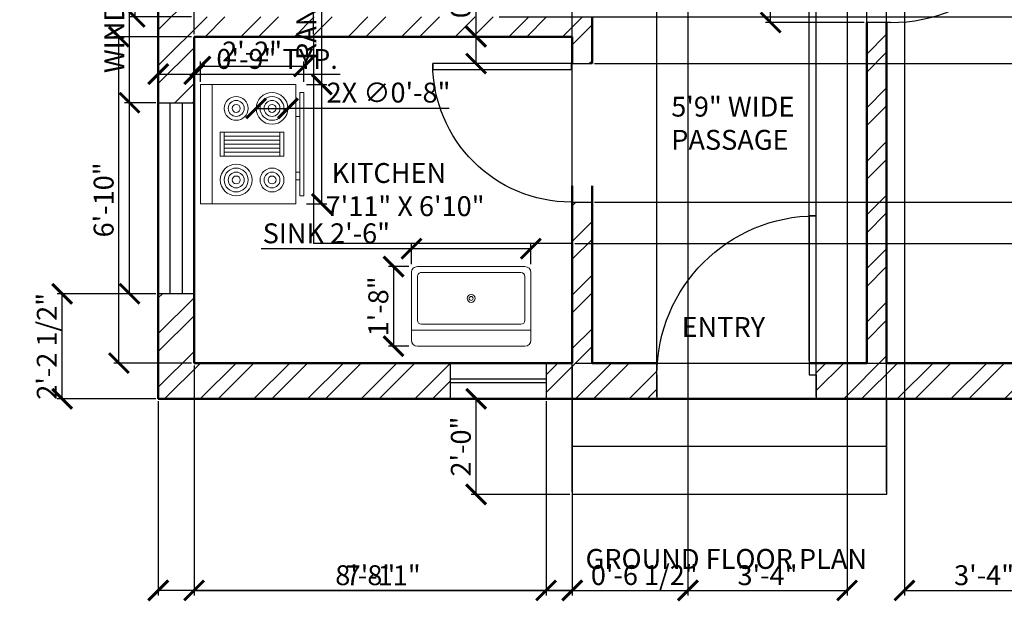
# Model space of a CAD drawing. Units: inches. Extents: x 683 to 1274, y 1901 to 2385.
# Tile 1 of 5: x 683 to 930, y 1901 to 2049. Entities that reach past the tile are written whole.
import ezdxf

# ---------------------------------------------------------------- set-up
doc = ezdxf.new("R2010")
doc.units = ezdxf.units.IN
for name, color, linetype, lineweight in [('A-AREA-IDEN', 3, 'Continuous', 25), ('A-EQPM', 2, 'Continuous', 18), ('A-FLOR-CASE', 2, 'Continuous', 25), ('A-FLOR-FIXT', 2, 'Continuous', 18), ('A-FLOR-STRS', 7, 'Continuous', 25), ('A-WALL-PATT', 8, 'Continuous', 13), ('DIM', 3, 'Continuous', 18), ('DOORS', 4, 'Continuous', 25), ('TEXT', 1, 'Continuous', 25), ('VENTILATOR', 11, 'Continuous', 25), ('walls', 6, 'Continuous', 50), ('WINDOWS', 30, 'Continuous', 25)]:
    doc.layers.add(name, color=color, linetype=linetype, lineweight=lineweight)
doc.styles.get("Standard").update_dxf_attribs({"font": 'arial.ttf'})
doc.dimstyles.new('ISO-25', dxfattribs={"dimtxt": 5, "dimasz": 5, "dimexe": 1.25, "dimexo": 0.625, "dimtad": 1, "dimdec": 1, "dimlunit": 4, "dimtxsty": 'Standard', "dimblk": 'ARCHTICK', "dimcen": 2.5, "dimadec": 0, "dimazin": 0, "dimtfac": 1, "dimtdec": 1, "dimtmove": 0, "dimatfit": 3, "dimfxl": 1, "dimarcsym": 0})

# ---------------------------------------------------------------- blocks, each defined once
blk = doc.blocks.new('Range-Oven - 30 in top')
for p, q in [((0, -3), (30, -3)), ((12, -6), (18, -6)), ((13, -20), (13, -6)), ((14, -6), (14, -20)), ((15, -20), (15, -6)), ((16, -6), (16, -20)), ((17, -20), (17, -6)), ((18, -20), (12, -20)), ((6, -24), (6, -25)), ((8, -25), (8, -24)), ((22, -25), (22, -24)), ((24, -24), (24, -25))]:
    blk.add_line(p, q)
for points in [[(0, -24), (0, 0), (30, 0), (30, -24)], [(12, -21), (12, -5), (18, -5), (18, -21)], [(2, -26), (2, -25), (28, -25), (28, -26)]]:
    blk.add_lwpolyline(points, close=True)
for centre, radius in [((6, -9), 4), ((6, -9), 3), ((6, -9), 2), ((24, -9), 3), ((24, -9), 2), ((6, -9), 1), ((24, -9), 1), ((24, -18), 4), ((6, -18), 3), ((6, -18), 2), ((6, -18), 1), ((24, -18), 3), ((24, -18), 2), ((24, -18), 1)]:
    blk.add_circle(centre, radius)
blk = doc.blocks.new('Sink-single - 30 in top')
blk.add_line((-15, -3.999996), (15, -3.999996))
for points in [[(-13.5, 0), (13.5, 0)], [(-15, -18.499996), (-15, -1.5)], [(15, -1.5), (15, -18.499996)], [(-13.5, -17.499996), (-13.5, -6.499996)], [(-12.5, -5.499996), (12.5, -5.499996)], [(13.5, -6.499996), (13.5, -17.499996)], [(12.5, -18.499996), (-12.5, -18.499996)], [(13.5, -19.999996), (-13.5, -19.999996)]]:
    blk.add_lwpolyline(points)
for radius in [1, 0.5]:
    blk.add_circle((0, -11.999996), radius)
for centre, radius, start, end in [((-13.5, -1.5), 1.5, 90, 180), ((13.5, -1.5), 1.5, 0, 90), ((-12.5, -6.499996), 1, 90, 180), ((12.5, -6.499996), 1, 0, 90), ((-13.5, -18.499996), 1.5, 180, 270), ((-12.5, -17.499996), 1, 180, 270), ((12.5, -17.499996), 1, 270, 0), ((13.5, -18.499996), 1.5, 270, 0)]:
    blk.add_arc(centre, radius, start, end)
blk = doc.blocks.new('VENTILATOR')
at = {"layer": 'VENTILATOR'}
for p, q in [((1084.96, 2166.43), (1093.96, 2166.43)), ((1084.96, 2142.43), (1084.96, 2166.43)), ((1088.96, 2142.43), (1088.96, 2166.43)), ((1089.96, 2166.43), (1089.96, 2142.43)), ((1093.96, 2166.43), (1093.96, 2142.43)), ((1093.96, 2142.43), (1084.96, 2142.43))]:
    blk.add_line(p, q, dxfattribs=at)
blk = doc.blocks.new('W2')
at = {"layer": 'WINDOWS'}
for p, q in [((1126.75, 2245.25), (1135.75, 2245.25)), ((1126.75, 2197.25), (1126.75, 2245.25)), ((1129.75, 2197.25), (1129.75, 2245.25)), ((1132.75, 2245.25), (1132.75, 2197.25)), ((1135.75, 2245.25), (1135.75, 2197.25)), ((1135.75, 2197.25), (1126.75, 2197.25))]:
    blk.add_line(p, q, dxfattribs=at)
blk = doc.blocks.new('*U18')
for p, q in [((0, 0), (0, -6)), ((40, 0), (40, -6))]:
    blk.add_line(p, q)
blk.add_lwpolyline([(0, 0), (0, 40), (1.75, 40), (1.75, 0)], close=True)
blk.add_arc((0, 0), 40, 0, 90)
blk = doc.blocks.new('_ArchTick')
at = {"color": 0, "linetype": 'ByBlock', "const_width": 0.15}
blk.add_lwpolyline([(-0.5, -0.5), (0.5, 0.5)], dxfattribs=at)
blk = doc.blocks.new('*D23')
at = {"layer": 'Defpoints', "color": 0, "transparency": 16777216}
for p in [(726.42, 2191.78), (711.49, 2049.78), (726.42, 2049.78)]:
    blk.add_point(p, dxfattribs=at)
at = {"layer": 'DIM', "color": 0, "lineweight": -2, "transparency": 16777216}
for p, q in [((725.79, 2191.78), (710.24, 2191.78)), ((711.49, 2191.78), (711.49, 2049.78)), ((725.79, 2049.78), (710.24, 2049.78))]:
    blk.add_line(p, q, dxfattribs=at)
at = {"layer": 'DIM', "color": 0, "lineweight": -2, "transparency": 16777216, "xscale": 5, "yscale": 5, "zscale": 5}
for p, rotation in [((711.49, 2191.78), 90), ((711.49, 2049.78), 270)]:
    blk.add_blockref('_ArchTick', p, dxfattribs=dict(at, rotation=rotation))
at = {"layer": 'DIM', "color": 0, "transparency": 16777216, "insert": (708.32, 2120.78), "char_height": 5, "attachment_point": 5, "rotation": 90}
blk.add_mtext('11\'-10"', dxfattribs=at)
blk = doc.blocks.new('*D24')
at = {"layer": 'Defpoints', "color": 0, "transparency": 16777216}
for p in [(707.52, 2044.78), (726.42, 2044.78), (726.42, 1962.78)]:
    blk.add_point(p, dxfattribs=at)
at = {"layer": 'DIM', "color": 0, "lineweight": -2, "transparency": 16777216}
for p, q in [((725.79, 2044.78), (706.27, 2044.78)), ((707.52, 1962.78), (707.52, 2044.78)), ((725.79, 1962.78), (706.27, 1962.78))]:
    blk.add_line(p, q, dxfattribs=at)
at = {"layer": 'DIM', "color": 0, "lineweight": -2, "transparency": 16777216, "xscale": 5, "yscale": 5, "zscale": 5}
for p, rotation in [((707.52, 2044.78), 90), ((707.52, 1962.78), 270)]:
    blk.add_blockref('_ArchTick', p, dxfattribs=dict(at, rotation=rotation))
at = {"layer": 'DIM', "color": 0, "transparency": 16777216, "insert": (704.34, 2003.78), "char_height": 5, "attachment_point": 5, "rotation": 90}
blk.add_mtext('6\'-10"', dxfattribs=at)
blk = doc.blocks.new('*D29')
at = {"layer": 'Defpoints', "color": 0, "transparency": 16777216}
for p in [(710.22, 2028.18), (717.42, 2028.18), (717.42, 1980.18)]:
    blk.add_point(p, dxfattribs=at)
at = {"layer": 'DIM', "color": 0, "lineweight": -2, "transparency": 16777216}
for p, q in [((710.22, 2028.18), (710.22, 2110.12)), ((716.79, 2028.18), (708.97, 2028.18)), ((710.22, 1980.18), (710.22, 2028.18)), ((716.79, 1980.18), (708.97, 1980.18))]:
    blk.add_line(p, q, dxfattribs=at)
at = {"layer": 'DIM', "color": 0, "lineweight": -2, "transparency": 16777216, "xscale": 5, "yscale": 5, "zscale": 5}
for p, rotation in [((710.22, 2028.18), 90), ((710.22, 1980.18), 270)]:
    blk.add_blockref('_ArchTick', p, dxfattribs=dict(at, rotation=rotation))
at = {"layer": 'DIM', "color": 0, "transparency": 16777216, "insert": (707.01, 2071.65), "char_height": 5, "attachment_point": 5, "rotation": 90}
blk.add_mtext('WINDOW W2 4\'-0" TYP.', dxfattribs=at)
blk = doc.blocks.new('*D30')
at = {"layer": 'Defpoints', "color": 0, "transparency": 16777216}
for p in [(726.42, 2035.38), (717.42, 2028.18), (726.42, 2028.18)]:
    blk.add_point(p, dxfattribs=at)
at = {"layer": 'DIM', "color": 0, "lineweight": -2, "transparency": 16777216}
for p, q in [((717.42, 2028.81), (717.42, 2036.63)), ((726.42, 2028.81), (726.42, 2036.63)), ((717.42, 2035.38), (726.42, 2035.38)), ((726.42, 2035.38), (763.15, 2035.38))]:
    blk.add_line(p, q, dxfattribs=at)
at = {"layer": 'DIM', "color": 0, "lineweight": -2, "transparency": 16777216, "xscale": 5, "yscale": 5, "zscale": 5, "rotation": 180}
blk.add_blockref('_ArchTick', (717.42, 2035.38), dxfattribs=at)
at = {"layer": 'DIM', "color": 0, "lineweight": -2, "transparency": 16777216, "xscale": 5, "yscale": 5, "zscale": 5}
blk.add_blockref('_ArchTick', (726.42, 2035.38), dxfattribs=at)
at = {"layer": 'DIM', "color": 0, "transparency": 16777216, "insert": (747.28, 2038.56), "char_height": 5, "attachment_point": 5}
blk.add_mtext('0\'-9" TYP.', dxfattribs=at)
blk = doc.blocks.new('*D33')
at = {"layer": 'Defpoints', "color": 0, "transparency": 16777216}
for p in [(754, 2032.78), (758.5, 2032.78), (754, 2002.78)]:
    blk.add_point(p, dxfattribs=at)
at = {"layer": 'DIM', "color": 0, "lineweight": -2, "transparency": 16777216}
for p, q in [((758.5, 2032.78), (758.5, 2078.84)), ((754.63, 2032.78), (759.75, 2032.78)), ((758.5, 2002.78), (758.5, 2032.78)), ((754.63, 2002.78), (759.75, 2002.78))]:
    blk.add_line(p, q, dxfattribs=at)
at = {"layer": 'DIM', "color": 0, "lineweight": -2, "transparency": 16777216, "xscale": 5, "yscale": 5, "zscale": 5}
for p, rotation in [((758.5, 2032.78), 90), ((758.5, 2002.78), 270)]:
    blk.add_blockref('_ArchTick', p, dxfattribs=dict(at, rotation=rotation))
at = {"layer": 'DIM', "color": 0, "transparency": 16777216, "insert": (755.29, 2058.31), "char_height": 5, "attachment_point": 5, "rotation": 90}
blk.add_mtext('RANGE 2\'-6"', dxfattribs=at)
blk = doc.blocks.new('*D34')
at = {"layer": 'Defpoints', "color": 0, "transparency": 16777216}
for p in [(728, 2037.28), (728, 2032.78), (754, 2032.78)]:
    blk.add_point(p, dxfattribs=at)
at = {"layer": 'DIM', "color": 0, "lineweight": -2, "transparency": 16777216}
for p, q in [((728, 2033.41), (728, 2038.53)), ((754, 2033.41), (754, 2038.53)), ((754, 2037.28), (728, 2037.28))]:
    blk.add_line(p, q, dxfattribs=at)
at = {"layer": 'DIM', "color": 0, "lineweight": -2, "transparency": 16777216, "xscale": 5, "yscale": 5, "zscale": 5, "rotation": 180}
blk.add_blockref('_ArchTick', (728, 2037.28), dxfattribs=at)
at = {"layer": 'DIM', "color": 0, "lineweight": -2, "transparency": 16777216, "xscale": 5, "yscale": 5, "zscale": 5}
blk.add_blockref('_ArchTick', (754, 2037.28), dxfattribs=at)
at = {"layer": 'DIM', "color": 0, "transparency": 16777216, "insert": (741, 2040.42), "char_height": 5, "attachment_point": 5}
blk.add_mtext('2\'-2"', dxfattribs=at)
blk = doc.blocks.new('*D35')
at = {"layer": 'Defpoints', "color": 0, "transparency": 16777216}
for p in [(781.03, 1991.52), (781.03, 1987.02), (811.03, 1987.02)]:
    blk.add_point(p, dxfattribs=at)
at = {"layer": 'DIM', "color": 0, "lineweight": -2, "transparency": 16777216}
for p, q in [((781.03, 1991.52), (743.27, 1991.52)), ((781.03, 1987.65), (781.03, 1992.77)), ((811.03, 1991.52), (781.03, 1991.52)), ((811.03, 1987.65), (811.03, 1992.77))]:
    blk.add_line(p, q, dxfattribs=at)
at = {"layer": 'DIM', "color": 0, "lineweight": -2, "transparency": 16777216, "xscale": 5, "yscale": 5, "zscale": 5, "rotation": 180}
blk.add_blockref('_ArchTick', (781.03, 1991.52), dxfattribs=at)
at = {"layer": 'DIM', "color": 0, "lineweight": -2, "transparency": 16777216, "xscale": 5, "yscale": 5, "zscale": 5}
blk.add_blockref('_ArchTick', (811.03, 1991.52), dxfattribs=at)
at = {"layer": 'DIM', "color": 0, "transparency": 16777216, "insert": (759.65, 1994.73), "char_height": 5, "attachment_point": 5}
blk.add_mtext('SINK 2\'-6"', dxfattribs=at)
blk = doc.blocks.new('*D36')
at = {"layer": 'Defpoints', "color": 0, "transparency": 16777216}
for p in [(781.03, 1987.02), (776.53, 1967.02), (781.03, 1967.02)]:
    blk.add_point(p, dxfattribs=at)
at = {"layer": 'DIM', "color": 0, "lineweight": -2, "transparency": 16777216}
for p, q in [((780.41, 1987.02), (775.28, 1987.02)), ((776.53, 1987.02), (776.53, 1967.02)), ((780.41, 1967.02), (775.28, 1967.02))]:
    blk.add_line(p, q, dxfattribs=at)
at = {"layer": 'DIM', "color": 0, "lineweight": -2, "transparency": 16777216, "xscale": 5, "yscale": 5, "zscale": 5}
for p, rotation in [((776.53, 1987.02), 90), ((776.53, 1967.02), 270)]:
    blk.add_blockref('_ArchTick', p, dxfattribs=dict(at, rotation=rotation))
at = {"layer": 'DIM', "color": 0, "transparency": 16777216, "insert": (773.35, 1977.02), "char_height": 5, "attachment_point": 5, "rotation": 90}
blk.add_mtext('1\'-8"', dxfattribs=at)
blk = doc.blocks.new('*D39')
at = {"layer": 'Defpoints', "color": 0, "transparency": 16777216}
for p in [(900.42, 2361.93), (821.42, 1929.78), (900.42, 1929.78)]:
    blk.add_point(p, dxfattribs=at)
at = {"layer": 'DIM', "color": 0, "lineweight": -2, "transparency": 16777216}
for p, q in [((821.42, 1930.41), (821.42, 2363.18)), ((900.42, 1930.41), (900.42, 2363.18)), ((821.42, 2361.93), (900.42, 2361.93))]:
    blk.add_line(p, q, dxfattribs=at)
at = {"layer": 'DIM', "color": 0, "lineweight": -2, "transparency": 16777216, "xscale": 5, "yscale": 5, "zscale": 5, "rotation": 180}
blk.add_blockref('_ArchTick', (821.42, 2361.93), dxfattribs=at)
at = {"layer": 'DIM', "color": 0, "lineweight": -2, "transparency": 16777216, "xscale": 5, "yscale": 5, "zscale": 5}
blk.add_blockref('_ArchTick', (900.42, 2361.93), dxfattribs=at)
at = {"layer": 'DIM', "color": 0, "transparency": 16777216, "insert": (860.92, 2365.11), "char_height": 5, "attachment_point": 5}
blk.add_mtext('6\'-7"', dxfattribs=at)
blk = doc.blocks.new('*D40')
at = {"layer": 'Defpoints', "color": 0, "transparency": 16777216}
for p in [(797.27, 1953.78), (821.42, 1953.78), (821.42, 1929.78)]:
    blk.add_point(p, dxfattribs=at)
at = {"layer": 'DIM', "color": 0, "lineweight": -2, "transparency": 16777216}
for p, q in [((820.79, 1953.78), (796.02, 1953.78)), ((797.27, 1929.78), (797.27, 1953.78)), ((820.79, 1929.78), (796.02, 1929.78))]:
    blk.add_line(p, q, dxfattribs=at)
at = {"layer": 'DIM', "color": 0, "lineweight": -2, "transparency": 16777216, "xscale": 5, "yscale": 5, "zscale": 5}
for p, rotation in [((797.27, 1953.78), 90), ((797.27, 1929.78), 270)]:
    blk.add_blockref('_ArchTick', p, dxfattribs=dict(at, rotation=rotation))
at = {"layer": 'DIM', "color": 0, "transparency": 16777216, "insert": (794.09, 1941.78), "char_height": 5, "attachment_point": 5, "rotation": 90}
blk.add_mtext('2\'-0"', dxfattribs=at)
blk = doc.blocks.new('*D41')
at = {"layer": 'Defpoints', "color": 0, "transparency": 16777216}
for p in [(726.42, 1962.78), (821.42, 1962.78), (821.42, 1905.63)]:
    blk.add_point(p, dxfattribs=at)
at = {"layer": 'DIM', "color": 0, "lineweight": -2, "transparency": 16777216}
for p, q in [((726.42, 1962.16), (726.42, 1904.38)), ((821.42, 1962.16), (821.42, 1904.38)), ((726.42, 1905.63), (821.42, 1905.63))]:
    blk.add_line(p, q, dxfattribs=at)
at = {"layer": 'DIM', "color": 0, "lineweight": -2, "transparency": 16777216, "xscale": 5, "yscale": 5, "zscale": 5, "rotation": 180}
blk.add_blockref('_ArchTick', (726.42, 1905.63), dxfattribs=at)
at = {"layer": 'DIM', "color": 0, "lineweight": -2, "transparency": 16777216, "xscale": 5, "yscale": 5, "zscale": 5}
blk.add_blockref('_ArchTick', (821.42, 1905.63), dxfattribs=at)
at = {"layer": 'DIM', "color": 0, "transparency": 16777216, "insert": (773.92, 1908.77), "char_height": 5, "attachment_point": 5}
blk.add_mtext('7\'-11"', dxfattribs=at)
blk = doc.blocks.new('*D42')
at = {"layer": 'Defpoints', "color": 0, "transparency": 16777216}
for p in [(826.42, 2038.04), (826.42, 2003.23), (1053.57, 2003.23)]:
    blk.add_point(p, dxfattribs=at)
at = {"layer": 'DIM', "color": 0, "lineweight": -2, "transparency": 16777216}
for p, q in [((827.04, 2038.04), (1054.82, 2038.04)), ((1053.57, 2038.04), (1053.57, 2003.23)), ((827.04, 2003.23), (1054.82, 2003.23))]:
    blk.add_line(p, q, dxfattribs=at)
at = {"layer": 'DIM', "color": 0, "lineweight": -2, "transparency": 16777216, "xscale": 5, "yscale": 5, "zscale": 5}
for p, rotation in [((1053.57, 2038.04), 90), ((1053.57, 2003.23), 270)]:
    blk.add_blockref('_ArchTick', p, dxfattribs=dict(at, rotation=rotation))
at = {"layer": 'DIM', "color": 0, "transparency": 16777216, "insert": (1050.43, 2020.64), "char_height": 5, "attachment_point": 5, "rotation": 90}
blk.add_mtext('2\'-11"', dxfattribs=at)
blk = doc.blocks.new('*D44')
at = {"layer": 'Defpoints', "color": 0, "transparency": 16777216}
for p in [(882.7, 2361.93), (842.7, 1953.78), (882.7, 1953.78)]:
    blk.add_point(p, dxfattribs=at)
at = {"layer": 'DIM', "color": 0, "lineweight": -2, "transparency": 16777216}
for p, q in [((842.7, 1954.41), (842.7, 2363.18)), ((882.7, 1954.41), (882.7, 2363.18)), ((842.7, 2361.93), (882.7, 2361.93))]:
    blk.add_line(p, q, dxfattribs=at)
at = {"layer": 'DIM', "color": 0, "lineweight": -2, "transparency": 16777216, "xscale": 5, "yscale": 5, "zscale": 5, "rotation": 180}
blk.add_blockref('_ArchTick', (842.7, 2361.93), dxfattribs=at)
at = {"layer": 'DIM', "color": 0, "lineweight": -2, "transparency": 16777216, "xscale": 5, "yscale": 5, "zscale": 5}
blk.add_blockref('_ArchTick', (882.7, 2361.93), dxfattribs=at)
at = {"layer": 'DIM', "color": 0, "transparency": 16777216, "insert": (862.7, 2365.11), "char_height": 5, "attachment_point": 5}
blk.add_mtext('3\'-4"', dxfattribs=at)
blk = doc.blocks.new('*D45')
at = {"layer": 'Defpoints', "color": 0, "transparency": 16777216}
for p in [(850.48, 2191.78), (890.48, 2191.78), (890.48, 1905.63)]:
    blk.add_point(p, dxfattribs=at)
at = {"layer": 'DIM', "color": 0, "lineweight": -2, "transparency": 16777216}
for p, q in [((850.48, 2191.16), (850.48, 1904.38)), ((890.48, 2191.16), (890.48, 1904.38)), ((850.48, 1905.63), (890.48, 1905.63))]:
    blk.add_line(p, q, dxfattribs=at)
at = {"layer": 'DIM', "color": 0, "lineweight": -2, "transparency": 16777216, "xscale": 5, "yscale": 5, "zscale": 5, "rotation": 180}
blk.add_blockref('_ArchTick', (850.48, 1905.63), dxfattribs=at)
at = {"layer": 'DIM', "color": 0, "lineweight": -2, "transparency": 16777216, "xscale": 5, "yscale": 5, "zscale": 5}
blk.add_blockref('_ArchTick', (890.48, 1905.63), dxfattribs=at)
at = {"layer": 'DIM', "color": 0, "transparency": 16777216, "insert": (870.48, 1908.81), "char_height": 5, "attachment_point": 5}
blk.add_mtext('3\'-4"', dxfattribs=at)
blk = doc.blocks.new('*D46')
at = {"layer": 'Defpoints', "color": 0, "transparency": 16777216}
for p in [(904.89, 2191.78), (944.89, 2191.78), (944.89, 1905.63)]:
    blk.add_point(p, dxfattribs=at)
at = {"layer": 'DIM', "color": 0, "lineweight": -2, "transparency": 16777216}
for p, q in [((904.89, 2191.16), (904.89, 1904.38)), ((944.89, 2191.16), (944.89, 1904.38)), ((904.89, 1905.63), (944.89, 1905.63))]:
    blk.add_line(p, q, dxfattribs=at)
at = {"layer": 'DIM', "color": 0, "lineweight": -2, "transparency": 16777216, "xscale": 5, "yscale": 5, "zscale": 5, "rotation": 180}
blk.add_blockref('_ArchTick', (904.89, 1905.63), dxfattribs=at)
at = {"layer": 'DIM', "color": 0, "lineweight": -2, "transparency": 16777216, "xscale": 5, "yscale": 5, "zscale": 5}
blk.add_blockref('_ArchTick', (944.89, 1905.63), dxfattribs=at)
at = {"layer": 'DIM', "color": 0, "transparency": 16777216, "insert": (924.89, 1908.81), "char_height": 5, "attachment_point": 5}
blk.add_mtext('3\'-4"', dxfattribs=at)
blk = doc.blocks.new('*D47')
at = {"layer": 'Defpoints', "color": 0, "transparency": 16777216}
for p in [(871.27, 2088.36), (895.42, 2088.36), (895.42, 2048.36)]:
    blk.add_point(p, dxfattribs=at)
at = {"layer": 'DIM', "color": 0, "lineweight": -2, "transparency": 16777216}
for p, q in [((894.79, 2088.36), (870.02, 2088.36)), ((871.27, 2048.36), (871.27, 2088.36)), ((894.79, 2048.36), (870.02, 2048.36))]:
    blk.add_line(p, q, dxfattribs=at)
at = {"layer": 'DIM', "color": 0, "lineweight": -2, "transparency": 16777216, "xscale": 5, "yscale": 5, "zscale": 5}
for p, rotation in [((871.27, 2088.36), 90), ((871.27, 2048.36), 270)]:
    blk.add_blockref('_ArchTick', p, dxfattribs=dict(at, rotation=rotation))
at = {"layer": 'DIM', "color": 0, "transparency": 16777216, "insert": (868.09, 2068.36), "char_height": 5, "attachment_point": 5, "rotation": 90}
blk.add_mtext('3\'-4"', dxfattribs=at)
blk = doc.blocks.new('*D49')
at = {"layer": 'Defpoints', "color": 0, "transparency": 16777216}
for p in [(802.42, 2085.78), (1053.57, 2085.78), (802.42, 2049.78)]:
    blk.add_point(p, dxfattribs=at)
at = {"layer": 'DIM', "color": 0, "lineweight": -2, "transparency": 16777216}
for p, q in [((803.04, 2085.78), (1054.82, 2085.78)), ((1053.57, 2049.78), (1053.57, 2085.78)), ((803.04, 2049.78), (1054.82, 2049.78))]:
    blk.add_line(p, q, dxfattribs=at)
at = {"layer": 'DIM', "color": 0, "lineweight": -2, "transparency": 16777216, "xscale": 5, "yscale": 5, "zscale": 5}
for p, rotation in [((1053.57, 2085.78), 90), ((1053.57, 2049.78), 270)]:
    blk.add_blockref('_ArchTick', p, dxfattribs=dict(at, rotation=rotation))
at = {"layer": 'DIM', "color": 0, "transparency": 16777216, "insert": (1050.39, 2067.78), "char_height": 5, "attachment_point": 5, "rotation": 90}
blk.add_mtext('3\'-0"', dxfattribs=at)
blk = doc.blocks.new('*D56')
at = {"layer": 'Defpoints', "color": 0, "transparency": 16777216}
for p in [(693.27, 1980.18), (717.42, 1980.18), (717.42, 1953.78)]:
    blk.add_point(p, dxfattribs=at)
at = {"layer": 'DIM', "color": 0, "lineweight": -2, "transparency": 16777216}
for p, q in [((716.79, 1980.18), (692.02, 1980.18)), ((693.27, 1953.78), (693.27, 1980.18)), ((716.79, 1953.78), (692.02, 1953.78))]:
    blk.add_line(p, q, dxfattribs=at)
at = {"layer": 'DIM', "color": 0, "lineweight": -2, "transparency": 16777216, "xscale": 5, "yscale": 5, "zscale": 5}
for p, rotation in [((693.27, 1980.18), 90), ((693.27, 1953.78), 270)]:
    blk.add_blockref('_ArchTick', p, dxfattribs=dict(at, rotation=rotation))
at = {"layer": 'DIM', "color": 0, "transparency": 16777216, "insert": (690.06, 1966.98), "char_height": 5, "attachment_point": 5, "rotation": 90}
blk.add_mtext('2\'-2 1/2"', dxfattribs=at)
blk = doc.blocks.new('*D57')
at = {"layer": 'Defpoints', "color": 0, "transparency": 16777216}
for p in [(814.86, 1953.78), (821.42, 1953.78), (821.42, 1905.63)]:
    blk.add_point(p, dxfattribs=at)
at = {"layer": 'DIM', "color": 0, "lineweight": -2, "transparency": 16777216}
for p, q in [((814.86, 1953.16), (814.86, 1904.38)), ((821.42, 1953.16), (821.42, 1904.38)), ((814.86, 1905.63), (821.42, 1905.63)), ((821.42, 1905.63), (852.61, 1905.63))]:
    blk.add_line(p, q, dxfattribs=at)
at = {"layer": 'DIM', "color": 0, "lineweight": -2, "transparency": 16777216, "xscale": 5, "yscale": 5, "zscale": 5, "rotation": 180}
blk.add_blockref('_ArchTick', (814.86, 1905.63), dxfattribs=at)
at = {"layer": 'DIM', "color": 0, "lineweight": -2, "transparency": 16777216, "xscale": 5, "yscale": 5, "zscale": 5}
blk.add_blockref('_ArchTick', (821.42, 1905.63), dxfattribs=at)
at = {"layer": 'DIM', "color": 0, "transparency": 16777216, "insert": (839.52, 1908.84), "char_height": 5, "attachment_point": 5}
blk.add_mtext('0\'-6 1/2"', dxfattribs=at)
blk = doc.blocks.new('*D58')
at = {"layer": 'Defpoints', "color": 0, "transparency": 16777216}
for p in [(756.42, 2361.93), (726.42, 2044.78), (756.42, 2044.78)]:
    blk.add_point(p, dxfattribs=at)
at = {"layer": 'DIM', "color": 0, "lineweight": -2, "transparency": 16777216}
for p, q in [((726.42, 2045.41), (726.42, 2363.18)), ((756.42, 2045.41), (756.42, 2363.18)), ((726.42, 2361.93), (756.42, 2361.93))]:
    blk.add_line(p, q, dxfattribs=at)
at = {"layer": 'DIM', "color": 0, "lineweight": -2, "transparency": 16777216, "xscale": 5, "yscale": 5, "zscale": 5, "rotation": 180}
blk.add_blockref('_ArchTick', (726.42, 2361.93), dxfattribs=at)
at = {"layer": 'DIM', "color": 0, "lineweight": -2, "transparency": 16777216, "xscale": 5, "yscale": 5, "zscale": 5}
blk.add_blockref('_ArchTick', (756.42, 2361.93), dxfattribs=at)
at = {"layer": 'DIM', "color": 0, "transparency": 16777216, "insert": (741.42, 2365.11), "char_height": 5, "attachment_point": 5}
blk.add_mtext('2\'-6"', dxfattribs=at)
blk = doc.blocks.new('*D59')
at = {"layer": 'Defpoints', "color": 0, "transparency": 16777216}
for p in [(821.42, 1992.78), (821.42, 1962.78), (1053.57, 1962.78)]:
    blk.add_point(p, dxfattribs=at)
at = {"layer": 'DIM', "color": 0, "lineweight": -2, "transparency": 16777216}
for p, q in [((822.04, 1992.78), (1054.82, 1992.78)), ((1053.57, 1992.78), (1053.57, 1962.78)), ((822.04, 1962.78), (1054.82, 1962.78))]:
    blk.add_line(p, q, dxfattribs=at)
at = {"layer": 'DIM', "color": 0, "lineweight": -2, "transparency": 16777216, "xscale": 5, "yscale": 5, "zscale": 5}
for p, rotation in [((1053.57, 1992.78), 90), ((1053.57, 1962.78), 270)]:
    blk.add_blockref('_ArchTick', p, dxfattribs=dict(at, rotation=rotation))
at = {"layer": 'DIM', "color": 0, "transparency": 16777216, "insert": (1050.39, 1977.78), "char_height": 5, "attachment_point": 5, "rotation": 90}
blk.add_mtext('2\'-6"', dxfattribs=at)
blk = doc.blocks.new('*D61')
at = {"layer": 'Defpoints', "color": 0, "transparency": 16777216}
for p in [(895.42, 2361.93), (880.95, 1962.78), (895.42, 1962.78)]:
    blk.add_point(p, dxfattribs=at)
at = {"layer": 'DIM', "color": 0, "lineweight": -2, "transparency": 16777216}
for p, q in [((880.95, 1963.41), (880.95, 2363.18)), ((895.42, 1963.41), (895.42, 2363.18)), ((880.95, 2361.93), (895.42, 2361.93)), ((895.42, 2361.93), (926.14, 2361.93))]:
    blk.add_line(p, q, dxfattribs=at)
at = {"layer": 'DIM', "color": 0, "lineweight": -2, "transparency": 16777216, "xscale": 5, "yscale": 5, "zscale": 5, "rotation": 180}
blk.add_blockref('_ArchTick', (880.95, 2361.93), dxfattribs=at)
at = {"layer": 'DIM', "color": 0, "lineweight": -2, "transparency": 16777216, "xscale": 5, "yscale": 5, "zscale": 5}
blk.add_blockref('_ArchTick', (895.42, 2361.93), dxfattribs=at)
at = {"layer": 'DIM', "color": 0, "transparency": 16777216, "insert": (913.28, 2365.14), "char_height": 5, "attachment_point": 5}
blk.add_mtext('1\'-2 1/2"', dxfattribs=at)
blk = doc.blocks.new('*D62')
at = {"layer": 'Defpoints', "color": 0, "transparency": 16777216}
for p in [(717.42, 1953.78), (821.42, 1929.78), (717.42, 1905.63)]:
    blk.add_point(p, dxfattribs=at)
at = {"layer": 'DIM', "color": 0, "lineweight": -2, "transparency": 16777216}
for p, q in [((717.42, 1953.16), (717.42, 1904.38)), ((821.42, 1929.16), (821.42, 1904.38)), ((821.42, 1905.63), (717.42, 1905.63))]:
    blk.add_line(p, q, dxfattribs=at)
at = {"layer": 'DIM', "color": 0, "lineweight": -2, "transparency": 16777216, "xscale": 5, "yscale": 5, "zscale": 5, "rotation": 180}
blk.add_blockref('_ArchTick', (717.42, 1905.63), dxfattribs=at)
at = {"layer": 'DIM', "color": 0, "lineweight": -2, "transparency": 16777216, "xscale": 5, "yscale": 5, "zscale": 5}
blk.add_blockref('_ArchTick', (821.42, 1905.63), dxfattribs=at)
at = {"layer": 'DIM', "color": 0, "transparency": 16777216, "insert": (769.42, 1908.81), "char_height": 5, "attachment_point": 5}
blk.add_mtext('8\'-8"', dxfattribs=at)
blk = doc.blocks.new('*D66')
at = {"layer": 'Defpoints', "color": 0, "transparency": 16777216}
for p in [(797.27, 2044.78), (821.42, 2044.78), (821.42, 2038.04)]:
    blk.add_point(p, dxfattribs=at)
at = {"layer": 'DIM', "color": 0, "lineweight": -2, "transparency": 16777216}
for p, q in [((797.27, 2044.78), (797.27, 2075.97)), ((820.79, 2044.78), (796.02, 2044.78)), ((797.27, 2038.04), (797.27, 2044.78)), ((820.79, 2038.04), (796.02, 2038.04))]:
    blk.add_line(p, q, dxfattribs=at)
at = {"layer": 'DIM', "color": 0, "lineweight": -2, "transparency": 16777216, "xscale": 5, "yscale": 5, "zscale": 5}
for p, rotation in [((797.27, 2044.78), 90), ((797.27, 2038.04), 270)]:
    blk.add_blockref('_ArchTick', p, dxfattribs=dict(at, rotation=rotation))
at = {"layer": 'DIM', "color": 0, "transparency": 16777216, "insert": (794.06, 2062.88), "char_height": 5, "attachment_point": 5, "rotation": 90}
blk.add_mtext('0\'-6 1/2"', dxfattribs=at)
blk = doc.blocks.new('*D71')
at = {"layer": 'Defpoints', "color": 0, "transparency": 16777216}
for p in [(742, 2026.78), (750, 2026.78)]:
    blk.add_point(p, dxfattribs=at)
at = {"layer": 'DIM', "color": 0, "lineweight": -2, "transparency": 16777216}
for p in [(742, 2026.78), (790.54, 2026.78)]:
    blk.add_line(p, (750, 2026.78), dxfattribs=at)
at = {"layer": 'DIM', "color": 0, "lineweight": -2, "transparency": 16777216, "xscale": 5, "yscale": 5, "zscale": 5}
for p, rotation in [((742, 2026.78), 359.9946714925211), ((750, 2026.78), 179.994671492521)]:
    blk.add_blockref('_ArchTick', p, dxfattribs=dict(at, rotation=rotation))
at = {"layer": 'DIM', "color": 0, "transparency": 16777216, "insert": (775.27, 2030.1), "char_height": 5, "attachment_point": 5, "rotation": 359.9947}
blk.add_mtext('2X ∅0\'-8"', dxfattribs=at)

msp = doc.modelspace()

# ---------------------------------------------------------------- hatches: boundary and pattern name
at = {"layer": 'A-WALL-PATT'}
h = msp.add_hatch(dxfattribs=at)
h.set_pattern_fill('ANSI32', color=256)
h.paths.add_polyline_path([(717.42, 2337.78), (717.42, 2300.95), (726.42, 2300.95), (726.42, 2328.78), (895.42, 2328.78), (895.42, 2196.78), (890.48, 2196.78), (890.48, 2191.78), (904.89, 2191.78), (904.89, 2196.78), (900.42, 2196.78), (900.42, 2328.78), (1020.42, 2328.78), (1020.42, 2303.09), (1029.42, 2303.09), (1029.42, 2337.78)])
h.paths.add_polyline_path([(1020.42, 2196.78), (944.89, 2196.78), (944.89, 2191.78), (967.42, 2191.78), (967.42, 2184.95), (972.42, 2184.95), (972.42, 2191.78), (1020.42, 2191.78), (1020.42, 2129.51), (1029.42, 2129.51), (1029.42, 2243.09), (1020.42, 2243.09)])
h.paths.add_polyline_path([(1029.42, 2105.51), (1020.42, 2105.51), (1020.42, 2100.78), (972.42, 2100.78), (972.42, 2150.14), (967.42, 2150.14), (967.42, 2100.78), (895.42, 2100.78), (895.42, 2088.36), (900.42, 2088.36), (900.42, 2095.78), (1020.42, 2095.78), (1020.42, 1962.78), (1000.32, 1962.78), (1000.32, 1953.78), (1029.42, 1953.78)])
h.paths.add_polyline_path([(940.32, 1953.78), (940.32, 1962.78), (900.42, 1962.78), (900.42, 2048.36), (895.42, 2048.36), (895.42, 1962.78), (882.7, 1962.78), (882.7, 1959.78), (882.7, 1953.78)])
h.paths.add_polyline_path([(790.86, 1953.78), (790.86, 1962.78), (726.42, 1962.78), (726.42, 1980.18), (717.42, 1980.18), (717.42, 1953.78)])
h.paths.add_polyline_path([(842.7, 1953.78), (842.7, 1959.78, -0.01877), (842.81, 1962.78), (826.42, 1962.78), (826.42, 2003.23), (821.42, 2003.23), (821.42, 1962.78), (814.86, 1962.78), (814.86, 1953.78)])
h.paths.add_polyline_path([(726.42, 2196.78), (726.42, 2240.95), (717.42, 2240.95), (717.42, 2167.98), (726.42, 2167.98), (726.42, 2191.78), (850.48, 2191.78), (850.48, 2196.78)])
h = msp.add_hatch(dxfattribs=at)
h.set_pattern_fill('ANSI32', color=256)
h.paths.add_polyline_path([(726.42, 2119.98), (717.42, 2119.98), (717.42, 2028.18), (726.42, 2028.18), (726.42, 2044.78), (821.42, 2044.78), (821.42, 2038.04), (826.42, 2038.04), (826.42, 2049.78), (726.42, 2049.78)])

# ---------------------------------------------------------------- linework, layer by layer
at = {"layer": 'A-FLOR-CASE'}
for p in [(756.42, 2044.78), (821.42, 1992.78)]:
    msp.add_line(p, (756.42, 1992.78), dxfattribs=at)
at = {"layer": 'A-FLOR-STRS'}
for p, q in [((821.42, 1953.78), (821.42, 1929.78)), ((900.42, 1953.78), (900.42, 1929.78)), ((900.42, 1941.78), (821.42, 1941.78)), ((900.42, 1929.78), (821.42, 1929.78))]:
    msp.add_line(p, q, dxfattribs=at)
at = {"layer": 'walls'}
for p, q in [((717.42, 2337.78), (717.42, 1953.78)), ((826.42, 2038.04), (826.42, 2049.78)), ((895.42, 2048.36), (895.42, 1962.78)), ((900.42, 2048.36), (900.42, 1962.78)), ((726.42, 2044.78), (726.42, 1962.78)), ((821.42, 2044.78), (726.42, 2044.78)), ((821.42, 2044.78), (821.42, 2038.04)), ((821.42, 2007.28), (821.42, 1962.78)), ((826.42, 1962.78), (826.42, 2007.28)), ((821.42, 1962.78), (726.42, 1962.78)), ((842.81, 1962.78), (826.42, 1962.78)), ((895.42, 1962.78), (880.95, 1962.78)), ((1020.42, 1962.78), (900.42, 1962.78)), ((1029.42, 1953.78), (717.42, 1953.78))]:
    msp.add_line(p, q, dxfattribs=at)

# ---------------------------------------------------------------- block references
at = {"layer": 'A-EQPM', "rotation": 90}
msp.add_blockref('Range-Oven - 30 in top', (728, 2002.78), dxfattribs=at)
at = {"layer": 'A-FLOR-FIXT', "rotation": 180}
msp.add_blockref('Sink-single - 30 in top', (796.03, 1967.02), dxfattribs=at)
at = {"layer": 'DOORS', "rotation": 270}
msp.add_blockref('*U18', (901.42, 2088.36), dxfattribs=at)
at = {"layer": 'DOORS', "xscale": -0.8703088381272287, "yscale": 0.8703088381272287, "zscale": 0.8703088381272287, "rotation": 90}
msp.add_blockref('*U18', (821.2, 2038.04), dxfattribs=at)
at = {"layer": 'DOORS', "xscale": -1}
msp.add_blockref('*U18', (882.7, 1959.78), dxfattribs=at)
at = {"layer": 'VENTILATOR', "rotation": 270}
msp.add_blockref('VENTILATOR', (-1351.57, 3047.74), dxfattribs=at)
at = {"layer": 'WINDOWS'}
msp.add_blockref('W2', (-409.33, -217.06), dxfattribs=at)

# ---------------------------------------------------------------- texts
at = {"layer": 'A-AREA-IDEN', "char_height": 5, "attachment_point": 1}
for s, width, insert in [('{5\'9" WIDE PASSAGE}', 38.5091, (846.3, 2029.71)), ('{ KITCHEN  \\P7\'11" X 6\'10"}', 41.0348, (759.46, 2013.04))]:
    msp.add_mtext_dynamic_manual_height_columns(s, width=width, gutter_width=12.5, heights=[0], dxfattribs=dict(at, insert=insert))
at = {"layer": 'TEXT', "char_height": 5, "attachment_point": 1}
for s, width, insert in [('{ENTRY}', 7.8955, (848.9, 1974.34)), ('{GROUND FLOOR PLAN}', 78.6115, (824.77, 1916.05))]:
    msp.add_mtext_dynamic_manual_height_columns(s, width=width, gutter_width=12.5, heights=[0], dxfattribs=dict(at, insert=insert))

# ---------------------------------------------------------------- dimensions: what is measured, and where the dimension line sits
at = {"layer": 'DIM'}
for base, p1, p2, picture, middle in [((895.42, 2361.93), (880.95, 1962.78), (895.42, 1962.78), '*D61', (913.28, 2365.14)), ((756.42, 2361.93), (726.42, 2044.78), (756.42, 2044.78), '*D58', (741.42, 2365.11)), ((900.42, 2361.93), (821.42, 1929.78), (900.42, 1929.78), '*D39', (860.92, 2365.11)), ((882.7, 2361.93), (842.7, 1953.78), (882.7, 1953.78), '*D44', (862.7, 2365.11)), ((890.48, 1905.63), (850.48, 2191.78), (890.48, 2191.78), '*D45', (870.48, 1908.81)), ((944.89, 1905.63), (904.89, 2191.78), (944.89, 2191.78), '*D46', (924.89, 1908.81)), ((821.42, 1905.63), (726.42, 1962.78), (821.42, 1962.78), '*D41', (773.92, 1908.77)), ((717.42, 1905.63), (821.42, 1929.78), (717.42, 1953.78), '*D62', (769.42, 1908.81)), ((821.42, 1905.63), (814.86, 1953.78), (821.42, 1953.78), '*D57', (839.52, 1908.84))]:
    dim = msp.add_linear_dim(base=base, p1=p1, p2=p2, dimstyle='ISO-25', override={"dimdec": 1, "dimlfac": 1, "dimrnd": 0, "dimzin": 1, "dimdsep": 46, "dimlunit": 4, "dimfrac": 2}, dxfattribs=at)
    dim.commit()
    dim.dimension.update_dxf_attribs({"geometry": picture, "text_midpoint": middle})
for base, p1, p2, angle, override, picture, middle in [((711.49, 2049.78), (726.42, 2191.78), (726.42, 2049.78), 90, {"dimclrd": 0, "dimclre": 0, "dimclrt": 0}, '*D23', (708.32, 2120.78)), ((871.27, 2088.36), (895.42, 2048.36), (895.42, 2088.36), 90, {"dimdec": 1, "dimlfac": 1, "dimrnd": 0, "dimzin": 1, "dimdsep": 46, "dimlunit": 4, "dimfrac": 2}, '*D47', (868.09, 2068.36)), ((1053.57, 2085.78), (802.42, 2049.78), (802.42, 2085.78), 90, {"dimdec": 1, "dimlfac": 1, "dimrnd": 0, "dimzin": 1, "dimdsep": 46, "dimlunit": 4, "dimfrac": 2}, '*D49', (1050.39, 2067.78)), ((797.27, 2044.78), (821.42, 2038.04), (821.42, 2044.78), 90, {"dimdec": 1, "dimlfac": 1, "dimrnd": 0, "dimzin": 1, "dimdsep": 46, "dimlunit": 4, "dimfrac": 2}, '*D66', (794.06, 2062.88)), ((707.52, 2044.78), (726.42, 1962.78), (726.42, 2044.78), 90, {"dimclrd": 0, "dimclre": 0, "dimclrt": 0}, '*D24', (704.34, 2003.78)), ((728, 2037.28), (754, 2032.78), (728, 2032.78), 180, {"dimdec": 1, "dimlfac": 1, "dimrnd": 0, "dimzin": 1, "dimdsep": 46, "dimlunit": 4, "dimfrac": 2}, '*D34', (741, 2040.42)), ((1053.57, 2003.23), (826.42, 2038.04), (826.42, 2003.23), 90, {"dimdec": 1, "dimlfac": 1, "dimrnd": 0, "dimzin": 1, "dimdsep": 46, "dimlunit": 4, "dimfrac": 2}, '*D42', (1050.43, 2020.64)), ((1053.57, 1962.78), (821.42, 1992.78), (821.42, 1962.78), 90, {"dimdec": 1, "dimlfac": 1, "dimrnd": 0, "dimzin": 1, "dimdsep": 46, "dimlunit": 4, "dimfrac": 2}, '*D59', (1050.39, 1977.78)), ((776.53, 1967.02), (781.03, 1987.02), (781.03, 1967.02), 270, {"dimdec": 1, "dimlfac": 1, "dimrnd": 0, "dimzin": 1, "dimdsep": 46, "dimlunit": 4, "dimfrac": 2}, '*D36', (773.35, 1977.02)), ((693.27, 1980.18), (717.42, 1953.78), (717.42, 1980.18), 90, {"dimdec": 1, "dimlfac": 1, "dimrnd": 0, "dimzin": 1, "dimdsep": 46, "dimlunit": 4, "dimfrac": 2}, '*D56', (690.06, 1966.98)), ((797.27, 1953.78), (821.42, 1929.78), (821.42, 1953.78), 90, {"dimdec": 1, "dimlfac": 1, "dimrnd": 0, "dimzin": 1, "dimdsep": 46, "dimlunit": 4, "dimfrac": 2}, '*D40', (794.09, 1941.78))]:
    dim = msp.add_linear_dim(base=base, p1=p1, p2=p2, angle=angle, dimstyle='ISO-25', override=override, dxfattribs=at)
    dim.commit()
    dim.dimension.update_dxf_attribs({"geometry": picture, "text_midpoint": middle})
for base, p1, p2, angle, text, picture, middle in [((710.22, 2028.18), (717.42, 1980.18), (717.42, 2028.18), 90, 'WINDOW W2 <> TYP.', '*D29', (707.01, 2071.65)), ((758.5, 2032.78), (754, 2002.78), (754, 2032.78), 90, 'RANGE <>', '*D33', (755.29, 2058.31)), ((781.03, 1991.52), (811.03, 1987.02), (781.03, 1987.02), 180, 'SINK <>', '*D35', (759.65, 1994.73))]:
    dim = msp.add_linear_dim(base=base, p1=p1, p2=p2, angle=angle, text=text, dimstyle='ISO-25', override={"dimdec": 1, "dimlfac": 1, "dimrnd": 0, "dimzin": 1, "dimdsep": 46, "dimlunit": 4, "dimfrac": 2}, dxfattribs=at)
    dim.commit()
    dim.dimension.update_dxf_attribs({"geometry": picture, "text_midpoint": middle})
dim = msp.add_linear_dim(base=(726.42, 2035.38), p1=(717.42, 2028.18), p2=(726.42, 2028.18), text='<> TYP.', dimstyle='ISO-25', override={"dimdec": 1, "dimlfac": 1, "dimrnd": 0, "dimzin": 1, "dimdsep": 46, "dimlunit": 4, "dimfrac": 2}, dxfattribs=at)
dim.commit()
dim.dimension.update_dxf_attribs({"geometry": '*D30', "text_midpoint": (747.28, 2038.56)})
dim = msp.add_diameter_dim_2p(p1=(742, 2026.78), p2=(750, 2026.78), text='2X <>', dimstyle='ISO-25', override={"dimdec": 1, "dimlfac": 1, "dimrnd": 0, "dimzin": 1, "dimdsep": 46, "dimlunit": 4, "dimfrac": 2}, dxfattribs=at)
dim.commit()
dim.dimension.update_dxf_attribs({"geometry": '*D71', "text_midpoint": (775.27, 2026.78), "dimtype": 163})

doc.saveas('drawing.dxf')
